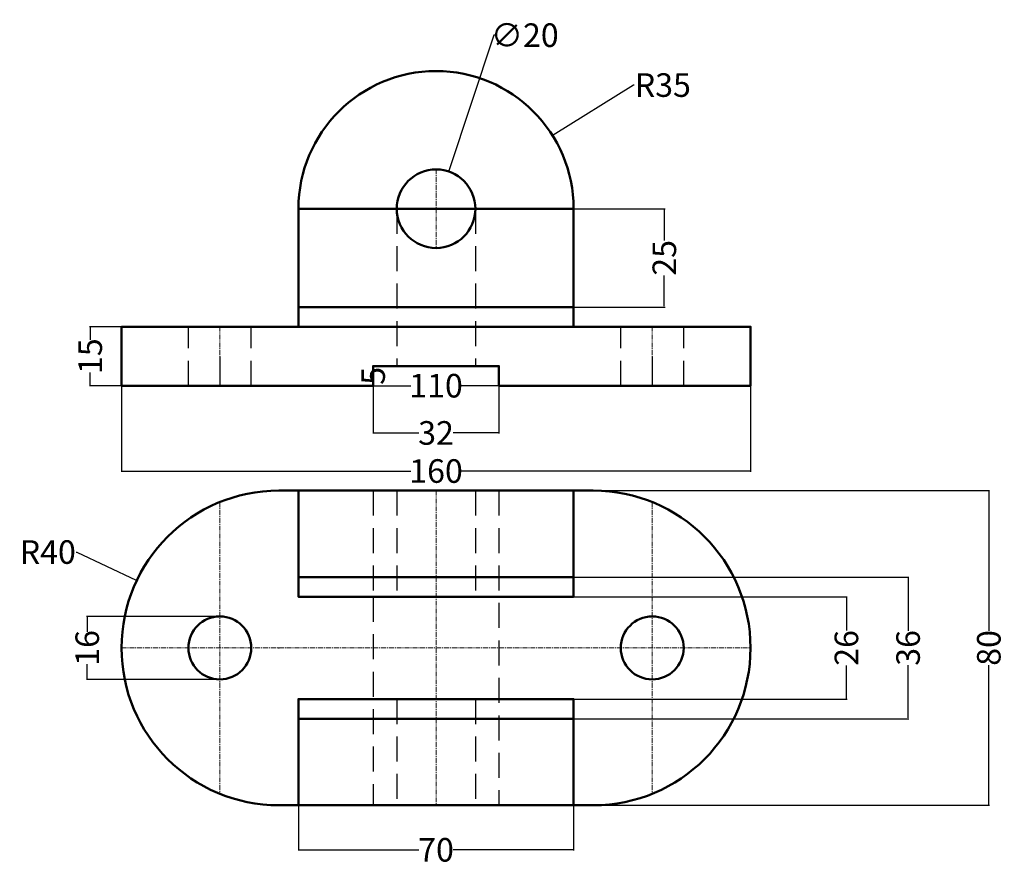
# Model space of a CAD drawing. Units: millimetres. Extents: x -1 to 250, y -3 to 212.
import ezdxf

# ---------------------------------------------------------------- set-up
doc = ezdxf.new("R2010")
doc.units = ezdxf.units.MM
doc.header["$MEASUREMENT"] = 0
doc.linetypes.add('CENTER', pattern=[2, 1.25, -0.25, 0.25, -0.25])
doc.linetypes.add('HIDDEN', pattern=[9.525, 6.35, -3.175])
for name, color, linetype, lineweight in [('M-CNTR', 1, 'CENTER', 18), ('M-DIMS', 3, 'Continuous', 25), ('M-HIDN', 2, 'HIDDEN', 25), ('M-OUTL', 7, 'Continuous', 50)]:
    doc.layers.add(name, color=color, linetype=linetype, lineweight=lineweight)
doc.styles.get("Standard").update_dxf_attribs({"font": 'arial.ttf'})
doc.dimstyles.get("Standard").update_dxf_attribs({"dimtxt": 6, "dimasz": 0.18, "dimexe": 0.18, "dimexo": 0.0625, "dimgap": 0.09, "dimtad": 0, "dimtoh": 1, "dimdec": 0, "dimzin": 0, "dimdsep": 46, "dimtxsty": 'Standard', "dimcen": 0.09, "dimadec": 0, "dimazin": 0, "dimtfac": 1, "dimtdec": 0, "dimtofl": 0, "dimtmove": 0, "dimatfit": 3, "dimfxl": 1, "dimtolj": 1, "dimtzin": 0, "dimarcsym": 0})

# ---------------------------------------------------------------- blocks, each defined once
blk = doc.blocks.new('*D1')
at = {"layer": 'Defpoints', "color": 0, "transparency": 16777216}
for p in [(140.08, 164.35), (140.08, 139.35), (163.15, 139.35)]:
    blk.add_point(p, dxfattribs=at)
at = {"layer": 'M-DIMS', "color": 0, "lineweight": -2, "transparency": 16777216}
for p, q in [((140.14, 164.35), (163.33, 164.35)), ((163.15, 164.17), (163.15, 156.31)), ((163.15, 139.53), (163.15, 147.39)), ((140.14, 139.35), (163.33, 139.35))]:
    blk.add_line(p, q, dxfattribs=at)
at = {"layer": 'M-DIMS', "color": 0, "transparency": 16777216}
for points in [[(163.12, 164.17), (163.18, 164.17), (163.15, 164.35)], [(163.12, 139.53), (163.18, 139.53), (163.15, 139.35)]]:
    blk.add_solid(points, dxfattribs=at)
at = {"layer": 'M-DIMS', "color": 0, "transparency": 16777216, "insert": (163.15, 151.85), "char_height": 6, "attachment_point": 5, "rotation": 90}
blk.add_mtext('\\A1;25', dxfattribs=at)
blk = doc.blocks.new('*D2')
at = {"layer": 'Defpoints', "color": 0, "transparency": 16777216}
for p in [(134.74, 182.92), (105.08, 164.35)]:
    blk.add_point(p, dxfattribs=at)
at = {"layer": 'M-DIMS', "color": 0, "lineweight": -2, "transparency": 16777216}
for p, q in [((155.31, 195.79), (134.9, 183.02)), ((155.49, 195.79), (155.31, 195.79)), ((104.99, 164.35), (105.17, 164.35)), ((105.08, 164.26), (105.08, 164.44))]:
    blk.add_line(p, q, dxfattribs=at)
at = {"layer": 'M-DIMS', "color": 0, "transparency": 16777216}
blk.add_solid([(134.88, 183.04), (134.91, 182.99), (134.74, 182.92)], dxfattribs=at)
at = {"layer": 'M-DIMS', "color": 0, "transparency": 16777216, "insert": (162.77, 195.79), "char_height": 6, "attachment_point": 5}
blk.add_mtext('\\A1;R35', dxfattribs=at)
blk = doc.blocks.new('*D3')
at = {"layer": 'Defpoints', "color": 0, "transparency": 16777216}
for p in [(108.25, 173.84), (101.91, 154.87)]:
    blk.add_point(p, dxfattribs=at)
at = {"layer": 'M-DIMS', "color": 0, "lineweight": -2, "transparency": 16777216}
for p, q in [((119.82, 208.48), (108.3, 174.01)), ((120, 208.48), (119.82, 208.48)), ((104.99, 164.35), (105.17, 164.35)), ((105.08, 164.26), (105.08, 164.44))]:
    blk.add_line(p, q, dxfattribs=at)
at = {"layer": 'M-DIMS', "color": 0, "transparency": 16777216}
blk.add_solid([(108.28, 174.02), (108.33, 174), (108.25, 173.84)], dxfattribs=at)
at = {"layer": 'M-DIMS', "color": 0, "transparency": 16777216, "insert": (127.65, 208.48), "char_height": 6, "attachment_point": 5}
blk.add_mtext('\\A1;∅20', dxfattribs=at)
blk = doc.blocks.new('*D4')
at = {"layer": 'Defpoints', "color": 0, "transparency": 16777216}
for p in [(25.08, 134.35), (17.1, 119.35), (25.08, 119.35)]:
    blk.add_point(p, dxfattribs=at)
at = {"layer": 'M-DIMS', "color": 0, "lineweight": -2, "transparency": 16777216}
for p, q in [((25.01, 134.35), (16.92, 134.35)), ((17.1, 134.17), (17.1, 130.98)), ((17.1, 119.53), (17.1, 122.72)), ((25.01, 119.35), (16.92, 119.35))]:
    blk.add_line(p, q, dxfattribs=at)
at = {"layer": 'M-DIMS', "color": 0, "transparency": 16777216}
for points in [[(17.07, 134.17), (17.13, 134.17), (17.1, 134.35)], [(17.07, 119.53), (17.13, 119.53), (17.1, 119.35)]]:
    blk.add_solid(points, dxfattribs=at)
at = {"layer": 'M-DIMS', "color": 0, "transparency": 16777216, "insert": (17.1, 126.85), "char_height": 6, "attachment_point": 5, "rotation": 90}
blk.add_mtext('\\A1;15', dxfattribs=at)
blk = doc.blocks.new('*D5')
at = {"layer": 'Defpoints', "color": 0, "transparency": 16777216}
for p in [(89.08, 119.35), (121.08, 119.35), (121.08, 107.34)]:
    blk.add_point(p, dxfattribs=at)
at = {"layer": 'M-DIMS', "color": 0, "lineweight": -2, "transparency": 16777216}
for p, q in [((89.08, 119.29), (89.08, 107.16)), ((121.08, 119.29), (121.08, 107.16)), ((89.26, 107.34), (100.72, 107.34)), ((120.9, 107.34), (109.43, 107.34))]:
    blk.add_line(p, q, dxfattribs=at)
at = {"layer": 'M-DIMS', "color": 0, "transparency": 16777216}
for points in [[(89.26, 107.37), (89.26, 107.31), (89.08, 107.34)], [(120.9, 107.37), (120.9, 107.31), (121.08, 107.34)]]:
    blk.add_solid(points, dxfattribs=at)
at = {"layer": 'M-DIMS', "color": 0, "transparency": 16777216, "insert": (105.08, 107.34), "char_height": 6, "attachment_point": 5}
blk.add_mtext('\\A1;32', dxfattribs=at)
blk = doc.blocks.new('*D6')
at = {"layer": 'Defpoints', "color": 0, "transparency": 16777216}
for p in [(89.08, 124.35), (89.08, 119.35), (89.08, 119.35)]:
    blk.add_point(p, dxfattribs=at)
at = {"layer": 'M-DIMS', "color": 0, "lineweight": -2, "transparency": 16777216}
for p, q in [((89.08, 124.17), (89.08, 123.93)), ((89.14, 124.35), (89.26, 124.35)), ((89.08, 119.53), (89.08, 119.77)), ((89.14, 119.35), (89.26, 119.35))]:
    blk.add_line(p, q, dxfattribs=at)
at = {"layer": 'M-DIMS', "color": 0, "transparency": 16777216}
for points in [[(89.05, 124.17), (89.11, 124.17), (89.08, 124.35)], [(89.05, 119.53), (89.11, 119.53), (89.08, 119.35)]]:
    blk.add_solid(points, dxfattribs=at)
at = {"layer": 'M-DIMS', "color": 0, "transparency": 16777216, "insert": (89.08, 121.85), "char_height": 6, "attachment_point": 5, "rotation": 90}
blk.add_mtext('\\A1;5', dxfattribs=at)
blk = doc.blocks.new('*D7')
at = {"layer": 'Defpoints', "color": 0, "transparency": 16777216}
for p in [(50.08, 126.85), (160.08, 126.85), (160.08, 119.35)]:
    blk.add_point(p, dxfattribs=at)
at = {"layer": 'M-DIMS', "color": 0, "lineweight": -2, "transparency": 16777216}
for p, q in [((50.08, 126.79), (50.08, 119.17)), ((160.08, 126.79), (160.08, 119.17)), ((50.26, 119.35), (98.65, 119.35)), ((159.9, 119.35), (111.5, 119.35))]:
    blk.add_line(p, q, dxfattribs=at)
at = {"layer": 'M-DIMS', "color": 0, "transparency": 16777216}
for points in [[(50.26, 119.38), (50.26, 119.32), (50.08, 119.35)], [(159.9, 119.38), (159.9, 119.32), (160.08, 119.35)]]:
    blk.add_solid(points, dxfattribs=at)
at = {"layer": 'M-DIMS', "color": 0, "transparency": 16777216, "insert": (105.08, 119.35), "char_height": 6, "attachment_point": 5}
blk.add_mtext('\\A1;110', dxfattribs=at)
blk = doc.blocks.new('*D8')
at = {"layer": 'Defpoints', "color": 0, "transparency": 16777216}
for p in [(25.08, 119.35), (185.08, 119.35), (185.08, 97.65)]:
    blk.add_point(p, dxfattribs=at)
at = {"layer": 'M-DIMS', "color": 0, "lineweight": -2, "transparency": 16777216}
for p, q in [((25.08, 119.29), (25.08, 97.47)), ((185.08, 119.29), (185.08, 97.47)), ((25.26, 97.65), (98.65, 97.65)), ((184.9, 97.65), (111.5, 97.65))]:
    blk.add_line(p, q, dxfattribs=at)
at = {"layer": 'M-DIMS', "color": 0, "transparency": 16777216}
for points in [[(25.26, 97.68), (25.26, 97.62), (25.08, 97.65)], [(184.9, 97.68), (184.9, 97.62), (185.08, 97.65)]]:
    blk.add_solid(points, dxfattribs=at)
at = {"layer": 'M-DIMS', "color": 0, "transparency": 16777216, "insert": (105.08, 97.65), "char_height": 6, "attachment_point": 5}
blk.add_mtext('\\A1;160', dxfattribs=at)
blk = doc.blocks.new('*D9')
at = {"layer": 'Defpoints', "color": 0, "transparency": 16777216}
for p in [(28.94, 69.83), (65.08, 52.67)]:
    blk.add_point(p, dxfattribs=at)
at = {"layer": 'M-DIMS', "color": 0, "lineweight": -2, "transparency": 16777216}
for p, q in [((13.56, 77.05), (13.74, 77.05)), ((13.74, 77.05), (28.78, 69.91)), ((64.99, 52.67), (65.17, 52.67)), ((65.08, 52.58), (65.08, 52.76))]:
    blk.add_line(p, q, dxfattribs=at)
at = {"layer": 'M-DIMS', "color": 0, "transparency": 16777216}
blk.add_solid([(28.79, 69.93), (28.77, 69.88), (28.94, 69.83)], dxfattribs=at)
at = {"layer": 'M-DIMS', "color": 0, "transparency": 16777216, "insert": (6.31, 77.05), "char_height": 6, "attachment_point": 5}
blk.add_mtext('\\A1;R40', dxfattribs=at)
blk = doc.blocks.new('*D10')
at = {"layer": 'Defpoints', "color": 0, "transparency": 16777216}
for p in [(50.08, 60.67), (16.35, 44.67), (50.08, 44.67)]:
    blk.add_point(p, dxfattribs=at)
at = {"layer": 'M-DIMS', "color": 0, "lineweight": -2, "transparency": 16777216}
for p, q in [((50.01, 60.67), (16.17, 60.67)), ((16.35, 60.49), (16.35, 56.77)), ((16.35, 44.85), (16.35, 48.57)), ((50.01, 44.67), (16.17, 44.67))]:
    blk.add_line(p, q, dxfattribs=at)
at = {"layer": 'M-DIMS', "color": 0, "transparency": 16777216}
for points in [[(16.32, 60.49), (16.38, 60.49), (16.35, 60.67)], [(16.32, 44.85), (16.38, 44.85), (16.35, 44.67)]]:
    blk.add_solid(points, dxfattribs=at)
at = {"layer": 'M-DIMS', "color": 0, "transparency": 16777216, "insert": (16.35, 52.67), "char_height": 6, "attachment_point": 5, "rotation": 90}
blk.add_mtext('\\A1;16', dxfattribs=at)
blk = doc.blocks.new('*D11')
at = {"layer": 'Defpoints', "color": 0, "transparency": 16777216}
for p in [(70.08, 12.67), (140.08, 12.67), (140.08, 1.33)]:
    blk.add_point(p, dxfattribs=at)
at = {"layer": 'M-DIMS', "color": 0, "lineweight": -2, "transparency": 16777216}
for p, q in [((70.08, 12.61), (70.08, 1.15)), ((140.08, 12.61), (140.08, 1.15)), ((70.26, 1.33), (100.72, 1.33)), ((139.9, 1.33), (109.43, 1.33))]:
    blk.add_line(p, q, dxfattribs=at)
at = {"layer": 'M-DIMS', "color": 0, "transparency": 16777216}
for points in [[(70.26, 1.36), (70.26, 1.3), (70.08, 1.33)], [(139.9, 1.36), (139.9, 1.3), (140.08, 1.33)]]:
    blk.add_solid(points, dxfattribs=at)
at = {"layer": 'M-DIMS', "color": 0, "transparency": 16777216, "insert": (105.08, 1.33), "char_height": 6, "attachment_point": 5}
blk.add_mtext('\\A1;70', dxfattribs=at)
blk = doc.blocks.new('*D12')
at = {"layer": 'Defpoints', "color": 0, "transparency": 16777216}
for p in [(140.08, 65.67), (140.08, 39.67), (209.47, 39.67)]:
    blk.add_point(p, dxfattribs=at)
at = {"layer": 'M-DIMS', "color": 0, "lineweight": -2, "transparency": 16777216}
for p, q in [((140.14, 65.67), (209.65, 65.67)), ((209.47, 65.49), (209.47, 57.11)), ((209.47, 39.85), (209.47, 48.23)), ((140.14, 39.67), (209.65, 39.67))]:
    blk.add_line(p, q, dxfattribs=at)
at = {"layer": 'M-DIMS', "color": 0, "transparency": 16777216}
for points in [[(209.44, 65.49), (209.5, 65.49), (209.47, 65.67)], [(209.44, 39.85), (209.5, 39.85), (209.47, 39.67)]]:
    blk.add_solid(points, dxfattribs=at)
at = {"layer": 'M-DIMS', "color": 0, "transparency": 16777216, "insert": (209.47, 52.67), "char_height": 6, "attachment_point": 5, "rotation": 90}
blk.add_mtext('\\A1;26', dxfattribs=at)
blk = doc.blocks.new('*D13')
at = {"layer": 'Defpoints', "color": 0, "transparency": 16777216}
for p in [(140.08, 70.67), (140.08, 34.67), (225.16, 34.67)]:
    blk.add_point(p, dxfattribs=at)
at = {"layer": 'M-DIMS', "color": 0, "lineweight": -2, "transparency": 16777216}
for p, q in [((140.14, 70.67), (225.34, 70.67)), ((225.16, 70.49), (225.16, 57.05)), ((225.16, 34.85), (225.16, 48.29)), ((140.14, 34.67), (225.34, 34.67))]:
    blk.add_line(p, q, dxfattribs=at)
at = {"layer": 'M-DIMS', "color": 0, "transparency": 16777216}
for points in [[(225.13, 70.49), (225.19, 70.49), (225.16, 70.67)], [(225.13, 34.85), (225.19, 34.85), (225.16, 34.67)]]:
    blk.add_solid(points, dxfattribs=at)
at = {"layer": 'M-DIMS', "color": 0, "transparency": 16777216, "insert": (225.16, 52.67), "char_height": 6, "attachment_point": 5, "rotation": 90}
blk.add_mtext('\\A1;36', dxfattribs=at)
blk = doc.blocks.new('*D14')
at = {"layer": 'Defpoints', "color": 0, "transparency": 16777216}
for p in [(140.08, 92.67), (140.08, 12.67), (245.7, 12.67)]:
    blk.add_point(p, dxfattribs=at)
at = {"layer": 'M-DIMS', "color": 0, "lineweight": -2, "transparency": 16777216}
for p, q in [((140.14, 92.67), (245.88, 92.67)), ((245.7, 92.49), (245.7, 57.05)), ((245.7, 12.85), (245.7, 48.29)), ((140.14, 12.67), (245.88, 12.67))]:
    blk.add_line(p, q, dxfattribs=at)
at = {"layer": 'M-DIMS', "color": 0, "transparency": 16777216}
for points in [[(245.67, 92.49), (245.73, 92.49), (245.7, 92.67)], [(245.67, 12.85), (245.73, 12.85), (245.7, 12.67)]]:
    blk.add_solid(points, dxfattribs=at)
at = {"layer": 'M-DIMS', "color": 0, "transparency": 16777216, "insert": (245.7, 52.67), "char_height": 6, "attachment_point": 5, "rotation": 90}
blk.add_mtext('\\A1;80', dxfattribs=at)

msp = doc.modelspace()

# ---------------------------------------------------------------- linework, layer by layer
at = {"layer": 'M-CNTR'}
for p, q in [((105.08, 174.35), (105.08, 154.35)), ((50.08, 134.35), (50.08, 119.35)), ((160.08, 134.35), (160.08, 119.35)), ((105.08, 92.67), (105.08, 12.67)), ((50.08, 89.75), (50.08, 15.59)), ((160.08, 89.75), (160.08, 15.59)), ((25.08, 52.67), (185.08, 52.67))]:
    msp.add_line(p, q, dxfattribs=at)
at = {"layer": 'M-HIDN'}
for p, q in [((95.08, 164.35), (95.08, 124.35)), ((115.08, 164.35), (115.08, 124.35)), ((42.08, 119.35), (42.08, 134.35)), ((58.08, 119.35), (58.08, 134.35)), ((152.08, 119.35), (152.08, 134.35)), ((168.08, 119.35), (168.08, 134.35)), ((95.08, 92.67), (95.08, 65.67)), ((115.08, 92.67), (115.08, 65.67)), ((121.08, 92.67), (121.08, 12.67)), ((95.08, 39.67), (95.08, 12.67)), ((115.08, 39.67), (115.08, 12.67))]:
    msp.add_line(p, q, dxfattribs=at)
msp.add_lwpolyline([(89.08, 92.67), (89.08, 65.67), (89.08, 12.67)], dxfattribs=at)
at = {"layer": 'M-OUTL'}
for p, q in [((70.08, 139.35), (140.08, 139.35)), ((70.08, 70.67), (140.08, 70.67)), ((70.08, 34.67), (140.08, 34.67))]:
    msp.add_line(p, q, dxfattribs=at)
msp.add_lwpolyline([(70.08, 164.35), (70.08, 134.35), (140.08, 134.35), (140.08, 164.35, 1), (70.08, 164.35), (140.08, 164.35)], format="xyb", dxfattribs=at)
for points in [[(89.08, 119.35), (25.08, 119.35), (25.08, 134.35), (70.08, 134.35)], [(89.08, 121.85), (89.08, 119.35), (89.08, 124.35), (121.08, 124.35), (121.08, 119.35), (185.08, 119.35), (185.08, 134.35), (140.08, 134.35)], [(70.08, 92.67), (70.08, 65.67), (140.08, 65.67), (140.08, 92.67)], [(140.08, 12.67), (140.08, 39.67), (70.08, 39.67), (70.08, 12.67)]]:
    msp.add_lwpolyline(points, dxfattribs=at)
msp.add_lwpolyline([(70.08, 92.67), (65.08, 92.67, 1), (65.08, 12.67), (70.08, 12.67), (140.08, 12.67), (145.08, 12.67, 1), (145.08, 92.67), (140.08, 92.67)], format="xyb", close=True, dxfattribs=at)
for centre, radius in [((105.08, 164.35), 10), ((50.08, 52.67), 8), ((160.08, 52.67), 8)]:
    msp.add_circle(centre, radius, dxfattribs=at)

# ---------------------------------------------------------------- dimensions: what is measured, and where the dimension line sits
at = {"layer": 'M-DIMS'}
dim = msp.add_diameter_dim_2p(p1=(101.91, 154.87), p2=(108.25, 173.84), dimstyle='Standard', override={"dimclrd": 0, "dimclre": 0, "dimclrt": 0}, dxfattribs=at)
dim.commit()
dim.dimension.update_dxf_attribs({"geometry": '*D3', "text_midpoint": (127.65, 208.48), "dimtype": 163})
for center, mpoint, picture, middle in [((105.08, 164.35), (134.74, 182.92), '*D2', (162.77, 195.79)), ((65.08, 52.67), (28.94, 69.83), '*D9', (6.31, 77.05))]:
    dim = msp.add_radius_dim(center=center, mpoint=mpoint, dimstyle='Standard', override={"dimclrd": 0, "dimclre": 0, "dimclrt": 0}, dxfattribs=at)
    dim.commit()
    dim.dimension.update_dxf_attribs({"geometry": picture, "text_midpoint": middle, "dimtype": 164})
for base, p1, p2, picture, middle in [((163.15, 139.35), (140.08, 164.35), (140.08, 139.35), '*D1', (163.15, 151.85)), ((17.1, 119.35), (25.08, 134.35), (25.08, 119.35), '*D4', (17.1, 126.85)), ((89.08, 119.35), (89.08, 124.35), (89.08, 119.35), '*D6', (89.08, 121.85)), ((245.7, 12.67), (140.08, 92.67), (140.08, 12.67), '*D14', (245.7, 52.67)), ((225.16, 34.67), (140.08, 70.67), (140.08, 34.67), '*D13', (225.16, 52.67)), ((209.47, 39.67), (140.08, 65.67), (140.08, 39.67), '*D12', (209.47, 52.67)), ((16.35, 44.67), (50.08, 60.67), (50.08, 44.67), '*D10', (16.35, 52.67))]:
    dim = msp.add_linear_dim(base=base, p1=p1, p2=p2, angle=90, dimstyle='Standard', override={"dimclrd": 0, "dimclre": 0, "dimclrt": 0}, dxfattribs=at)
    dim.commit()
    dim.dimension.update_dxf_attribs({"geometry": picture, "text_midpoint": middle})
for base, p1, p2, picture, middle in [((160.08, 119.35), (50.08, 126.85), (160.08, 126.85), '*D7', (105.08, 119.35)), ((185.08, 97.65), (25.08, 119.35), (185.08, 119.35), '*D8', (105.08, 97.65)), ((121.08, 107.34), (89.08, 119.35), (121.08, 119.35), '*D5', (105.08, 107.34)), ((140.08, 1.33), (70.08, 12.67), (140.08, 12.67), '*D11', (105.08, 1.33))]:
    dim = msp.add_linear_dim(base=base, p1=p1, p2=p2, dimstyle='Standard', override={"dimclrd": 0, "dimclre": 0, "dimclrt": 0}, dxfattribs=at)
    dim.commit()
    dim.dimension.update_dxf_attribs({"geometry": picture, "text_midpoint": middle})

doc.saveas('drawing.dxf')
